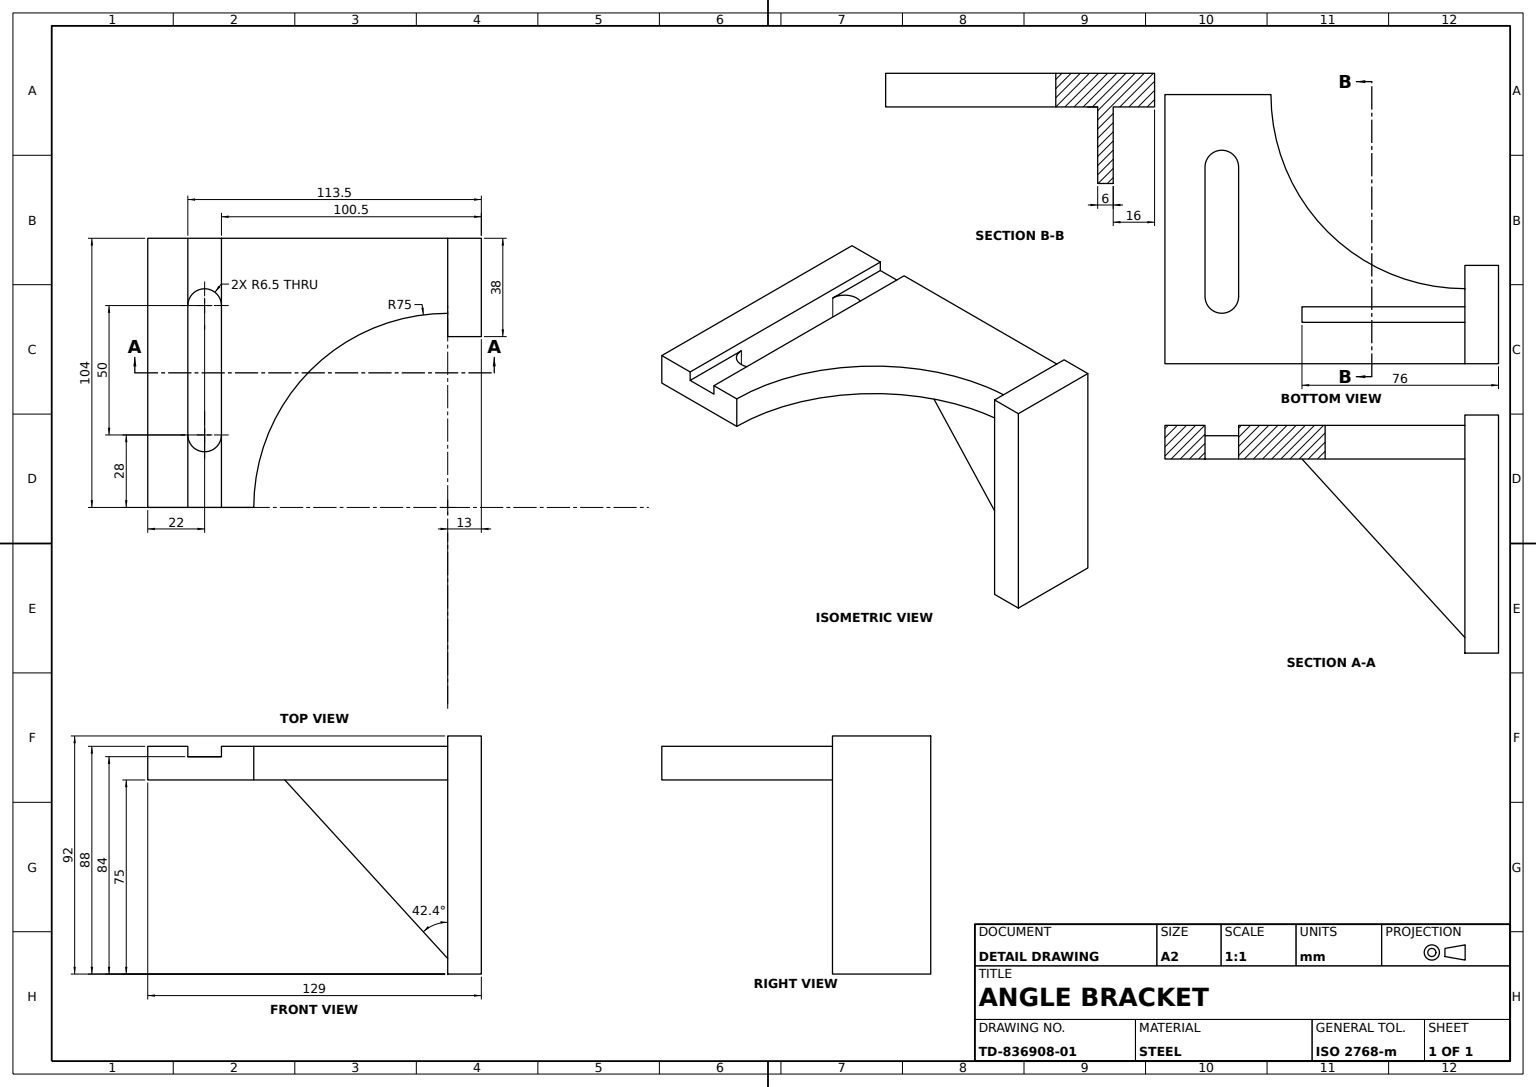
SolidWorks part; units mm, degrees
material "Plain Carbon Steel"
ref_plane "Front Plane" through (0, 0, 0) normal (0, 0, 1) x (1, 0, 0)
ref_plane "Top Plane" through (0, 0, 0) normal (0, 1, 0) x (1, 0, 0)
ref_plane "Right Plane" through (0, 0, 0) normal (1, 0, 0) x (0, 0, -1)
sketch "Base Plate Sketch" plane through (0, 0, 0) normal (0, 0, 1) x (1, 0, 0)
  line L0 (0, 0) -> (38, 0)
  line L1 (38, 0) -> (38, -92)
  line L2 (38, -92) -> (0, -92)
  line L3 (0, -92) -> (0, 0)
  dimension "D1" = 38
  dimension "D2" = 92
extrude "Base Plate" add sketch "Base Plate Sketch" along normal blind 13
sketch "Main Body Profile Sketch" plane through (0, 0, 0) normal (-1, 0, 0) x (0, 0, 1)
  line L0 (0, 0) -> (0, -92) construction
  line L1 (13, 0) -> (13, -92) construction
  line L2 (13, -4) -> (100.5, -4)
  line L3 (100.5, -4) -> (100.5, -8)
  line L4 (100.5, -8) -> (113.5, -8)
  line L5 (113.5, -8) -> (113.5, -4)
  line L6 (113.5, -4) -> (129, -4)
  line L7 (129, -4) -> (129, -17)
  line L8 (129, -17) -> (13, -17)
  line L9 (13, -17) -> (13, -4)
  line L10 (13, -92) -> (0, -92) construction
  dimension "D1" = 100.5
  dimension "D2" = 113.5
  dimension "D3" = 129
  dimension "D4" = 75
  dimension "D5" = 84
extrude "Main Body 104mm" add sketch "Main Body Profile Sketch" against normal blind 104
sketch "Curved Relief Sketch" plane through (0, -17, 0) normal (0, -1, 0) x (1, 0, 0)
  line L0 (104, 88) -> (104, 13)
  line L1 (104, 13) -> (29, 13)
  arc A0 (104, 88) -> (29, 13) centre (104, 13) ccw
  dimension "D1" = 75
extrude "Curved Relief Cut" cut sketch "Curved Relief Sketch" against normal blind 13
sketch "Slot Sketch" plane through (0, -17, 0) normal (0, -1, 0) x (1, 0, 0)
  line L0 (104, 129) -> (0, 129) construction
  line L1 (104, 88) -> (104, 129) construction
  line L2 (26, 113.5) -> (76, 113.5)
  line L3 (26, 100.5) -> (76, 100.5)
  arc A0 (76, 100.5) -> (76, 113.5) centre (76, 107) ccw
  arc A1 (26, 113.5) -> (26, 100.5) centre (26, 107) ccw
  dimension "D1" = 22
  dimension "D5" = 6.5
  dimension "D2" = 22
  dimension "D3" = 50
  dimension "D4" = 28
extrude "Slot Cut" cut sketch "Slot Sketch" against normal blind 13
sketch "Gusset Boss Sketch" plane through (0, 0, 0) normal (-1, 0, 0) x (0, 0, 1)
  line L0 (13, -17) -> (76, -17)
  line L1 (13, -17) -> (129, -17) construction
  line L2 (13, -17) -> (13, -86)
  line L3 (13, -17) -> (13, -92) construction
  line L4 (13, -86) -> (76, -17)
  line L5 (0, 0) -> (0, -92) construction
  line L6 (13, -92) -> (0, -92) construction
  dimension "D1" = 76
  dimension "D2" = 6
extrude "Gusset Boss 38mm" add sketch "Gusset Boss Sketch" against normal blind 38
sketch "Notch Cut A Sketch" plane through (38, 0, 0) normal (1, 0, 0) x (0, 0, -1)
  line L0 (-76, -17) -> (-13, -17)
  line L1 (-13, -17) -> (-13, -86)
  line L2 (-13, -86) -> (-76, -17)
extrude "Notch Cut A" cut sketch "Notch Cut A Sketch" against normal blind 16
sketch "Notch Cut B Sketch" plane through (0, 0, 0) normal (-1, 0, 0) x (0, 0, 1)
  line L0 (76, -17) -> (13, -86)
  line L1 (13, -86) -> (13, -17)
  line L2 (13, -17) -> (76, -17)
extrude "Notch Cut B" cut sketch "Notch Cut B Sketch" against normal blind 16
